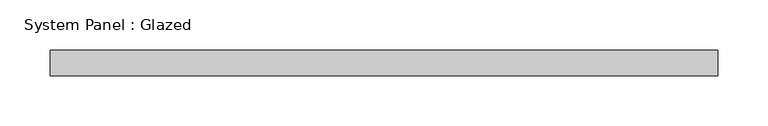
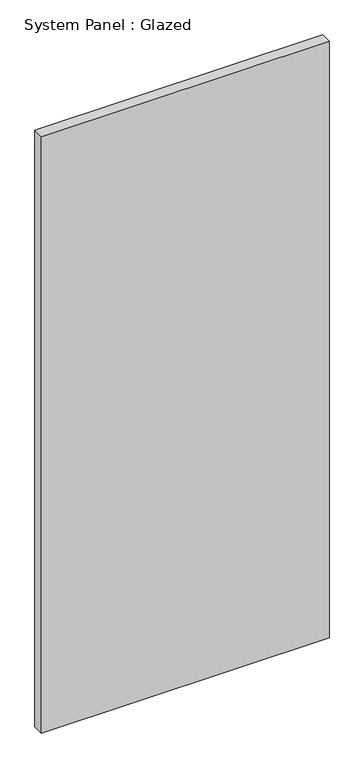
"""IFC4 building model written with IfcOpenShell, lengths in millimetres: plate geometry, System Panel : Glazed."""

from ifc_helpers import new_model, si_unit, origin, origin_with_axes, place, context, project, spatial, polyline, outline, extrude, source, transform, mapped, element, save


def system_panel_glazed_5bf0499b(model_context):
    return source(origin(), model_context, "Body", "SweptSolid", [
        extrude(outline(polyline([(333.375, 19.05), (-333.375, 19.05), (-333.375, 44.45), (333.375, 44.45), (333.375, 19.05)])), origin_with_axes(), (0.0, 0.0, 1.0), 1461.1134655),
    ])


if __name__ == "__main__":
    model = new_model("IFC4")
    model_context = context("Model", 3, world=origin())
    ifc_project = project(units=[si_unit("LENGTHUNIT", "METRE", prefix="MILLI")], contexts=[model_context])
    site = spatial("IfcSite", under=ifc_project)
    building = spatial("IfcBuilding", under=site)
    placement = place(None, origin())
    system_panel_glazed_shape = system_panel_glazed_5bf0499b(model_context)
    element("IfcPlate", 1, ObjectType="System Panel : Glazed", at=placement, inside=building, context=model_context, shape_type="MappedRepresentation", body=[
        mapped(system_panel_glazed_shape, transform((0.0, 0.0, 0.0), x_axis=(1.0, 0.0, 0.0), y_axis=(0.0, 1.0, 0.0), z_axis=(0.0, 0.0, 1.0))),
    ])
    save(model, "model.ifc")

# Revit data of these elements
# Type "System Panel : Glazed"
#   Construction Type Id = "GSP4R"
#   Analytic Construction = "1/8 in Pilkington single glazing"
#   Visual Light Transmittance = 0.9
#   Solar Heat Gain Coefficient = 0.86
#   Heat Transfer Coefficient (U) = 1.18115 BTU/(h·ft²·°F)
#   Define Thermal Properties by = 1
# Element 1 (IfcPlate, "System Panel : Glazed")
#   Materials on its faces: "Glass"
# Materials
#   "Glass": class "Glass", colour RGB 0 128 192, transparency 0.75, Description = "Soda Lime Glass", Cost = 0
